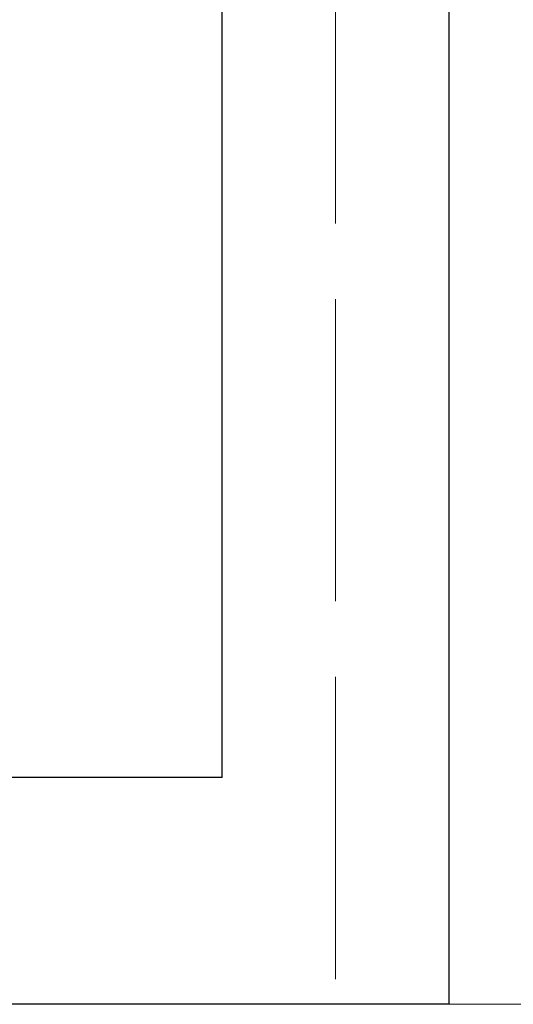
# Model space of a CAD drawing. Units: millimetres. Extents: x 595116 to 630915, y 909473 to 920225.
# Tile 105 of 134: x 629825 to 629845, y 919142 to 919181. Entities that reach past the tile are written whole.
import ezdxf

# ---------------------------------------------------------------- set-up
doc = ezdxf.new("R2010")
doc.units = ezdxf.units.MM
doc.linetypes.add('ACAD_ISO02W100', pattern=[15, 12, -3])
for name, color, linetype, lineweight in [('C-PROP', 7, 'Continuous', 25), ('C-PROP-REF', 240, 'ACAD_ISO02W100', 13), ('C-ROAD', 30, 'Continuous', 18)]:
    doc.layers.add(name, color=color, linetype=linetype, lineweight=lineweight)

msp = doc.modelspace()

# ---------------------------------------------------------------- linework, layer by layer
at = {"layer": 'C-PROP'}
for p, q in [((629833.541, 919150.928), (629833.541, 919345.928)), ((629842.541, 919345.928), (629842.541, 919141.928)), ((629833.541, 919150.928), (629809.541, 919150.928))]:
    msp.add_line(p, q, dxfattribs=at)
msp.add_lwpolyline([(629842.541, 919141.928), (629809.541, 919141.928)], dxfattribs=at)
at = {"layer": 'C-PROP-REF'}
msp.add_line((629838.041, 920084.928), (629838.041, 919141.928), dxfattribs=at)
at = {"layer": 'C-ROAD'}
msp.add_line((629842.541, 919141.928), (629943.895, 919141.928), dxfattribs=at)

doc.saveas('drawing.dxf')
